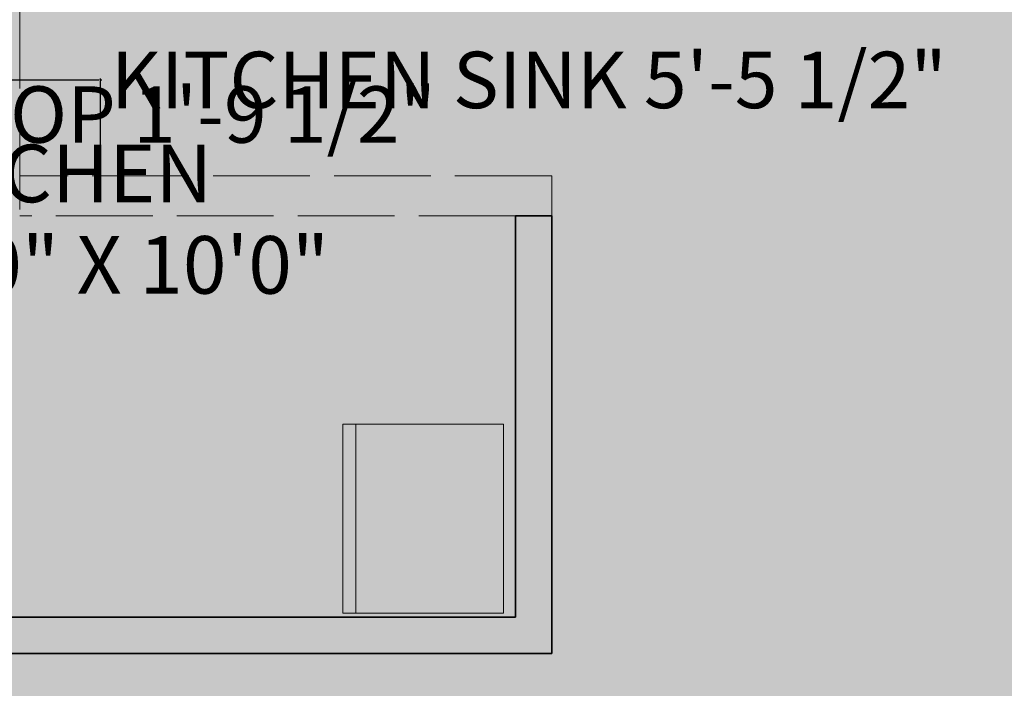
# Model space of a CAD drawing. Units: inches. Extents: x 1316 to 1777, y 813 to 1650.
# Tile 7 of 22: x 1445 to 1567, y 1237 to 1319. Entities that reach past the tile are written whole.
import ezdxf

# ---------------------------------------------------------------- set-up
doc = ezdxf.new("R2010")
doc.units = ezdxf.units.IN
doc.header["$MEASUREMENT"] = 0
doc.linetypes.add('ACAD_ISO02W100', pattern=[15, 12, -3])
for name, color, linetype, lineweight in [('A-ANNO-DIMS', 2, 'Continuous', 18), ('A-AREA-IDEN', 7, 'Continuous', 18), ('A-EQPM', 8, 'Continuous', 18), ('A-EQPM-PATT', 252, 'Continuous', 13), ('A-WALL-OVHD', 250, 'ACAD_ISO02W100', 18), ('A-WALL-PATT', 250, 'Continuous', 13), ('walls', 250, 'Continuous', 35)]:
    doc.layers.add(name, color=color, linetype=linetype, lineweight=lineweight)
doc.layers.add('A-FLOR-PATT', color=254, linetype='Continuous', lineweight=13, true_color=0xfeeab9)
doc.styles.get("Standard").update_dxf_attribs({"font": 'arial.ttf'})
doc.dimstyles.get("Standard").update_dxf_attribs({"dimtxt": 7, "dimasz": 0.18, "dimexe": 0.18, "dimexo": 0.0625, "dimgap": 0.09, "dimtad": 0, "dimtih": 1, "dimtoh": 1, "dimzin": 0, "dimdsep": 46, "dimlunit": 3, "dimtxsty": 'Standard', "dimcen": 0.09, "dimadec": 0, "dimazin": 0, "dimtfac": 1, "dimtofl": 0, "dimtmove": 0, "dimatfit": 3, "dimfxl": 1, "dimtolj": 1, "dimtzin": 0, "dimarcsym": 0})

# ---------------------------------------------------------------- blocks, each defined once
blk = doc.blocks.new('*D40')
at = {"layer": 'A-ANNO-DIMS', "color": 0, "lineweight": -2, "transparency": 16777216}
for p, q in [((1388.84, 1302.16), (1388.84, 1312.14)), ((1389.02, 1311.96), (1454.4, 1311.96)), ((1454.58, 1302.16), (1454.58, 1312.14)), ((1454.58, 1311.96), (1454.76, 1311.96))]:
    blk.add_line(p, q, dxfattribs=at)
at = {"layer": 'A-ANNO-DIMS', "color": 0, "transparency": 16777216}
for points in [[(1389.02, 1311.99), (1389.02, 1311.93), (1388.84, 1311.96)], [(1454.4, 1311.99), (1454.4, 1311.93), (1454.58, 1311.96)]]:
    blk.add_solid(points, dxfattribs=at)
at = {"layer": 'Defpoints', "color": 0, "transparency": 16777216}
for p in [(1454.58, 1311.96), (1388.84, 1302.1), (1454.58, 1302.1)]:
    blk.add_point(p, dxfattribs=at)
at = {"layer": 'A-ANNO-DIMS', "color": 0, "transparency": 16777216, "insert": (1507.74, 1311.96), "char_height": 7, "attachment_point": 5}
blk.add_mtext('\\A1;KITCHEN SINK 5\'-5 1/2"', dxfattribs=at)
blk = doc.blocks.new('*D42')
at = {"layer": 'A-ANNO-DIMS', "color": 0, "lineweight": -2, "transparency": 16777216}
for p, q in [((1388.61, 1310.85), (1388.61, 1307.49)), ((1410.21, 1310.85), (1410.21, 1307.49)), ((1388.79, 1307.67), (1410.03, 1307.67)), ((1410.21, 1307.67), (1410.39, 1307.67))]:
    blk.add_line(p, q, dxfattribs=at)
at = {"layer": 'A-ANNO-DIMS', "color": 0, "transparency": 16777216}
for points in [[(1388.79, 1307.7), (1388.79, 1307.64), (1388.61, 1307.67)], [(1410.03, 1307.7), (1410.03, 1307.64), (1410.21, 1307.67)]]:
    blk.add_solid(points, dxfattribs=at)
at = {"layer": 'Defpoints', "color": 0, "transparency": 16777216}
for p in [(1388.61, 1310.91), (1410.21, 1310.91), (1410.21, 1307.67)]:
    blk.add_point(p, dxfattribs=at)
at = {"layer": 'A-ANNO-DIMS', "color": 0, "transparency": 16777216, "insert": (1453.71, 1307.67), "char_height": 7, "attachment_point": 5}
blk.add_mtext('\\A1;COOKTOP 1\'-9 1/2"', dxfattribs=at)

msp = doc.modelspace()

# ---------------------------------------------------------------- hatches: boundary and pattern name
at = {"layer": 'A-EQPM-PATT'}
h = msp.add_hatch(color=256, dxfattribs=at)
h.dxf.hatch_style = 1
h.paths.add_polyline_path([(1504.59, 1269.305), (1486.26, 1269.305), (1486.26, 1245.841), (1504.59, 1245.841)])
h.paths.add_polyline_path([(1486.26, 1269.305), (1484.665, 1269.305), (1484.665, 1245.841), (1486.26, 1245.841)])
h = msp.add_hatch(color=256, dxfattribs=at)
h.dxf.hatch_style = 1
h.paths.add_polyline_path([(1506.155, 1265.562), (1504.59, 1265.562), (1504.59, 1250.33), (1506.155, 1250.33)])
at = {"layer": 'A-FLOR-PATT'}
h = msp.add_hatch(color=256, dxfattribs=at)
h.dxf.hatch_style = 1
h.paths.add_polyline_path([(1567.673, 1281.369), (1651.673, 1281.369), (1651.673, 1365.369), (1597.673, 1365.369), (1597.673, 1429.869), (1570.345, 1429.869), (1570.345, 1471.869), (1510.345, 1471.869), (1510.345, 1429.869), (1444.564, 1429.869), (1444.564, 1322.882), (1444.564, 1300.088), (1510.564, 1300.088), (1510.564, 1295.094), (1510.564, 1240.869), (1386.064, 1240.869), (1386.064, 1171.185), (1400.961, 1171.185), (1400.961, 1106.742), (1386.064, 1106.742), (1386.064, 1072.869), (1510.564, 1072.869), (1510.564, 1040.173), (1541.068, 1040.173, -0.367085), (1572.764, 1069.547), (1572.764, 1069.579), (1574.225, 1069.579), (1574.225, 1040.173), (1616.037, 1040.173), (1616.037, 1086.627), (1616.037, 1103.705), (1613.066, 1105.235), (1616.037, 1106.686), (1616.037, 1123.869), (1567.673, 1123.869)])
h.paths.add_polyline_path([(1508.987, 1198.018), (1511.117, 1198.018), (1511.117, 1200.148), (1532.595, 1200.148), (1532.595, 1198.018), (1534.725, 1198.018), (1534.725, 1176.008), (1530.465, 1176.008), (1530.465, 1176.718), (1513.247, 1176.718), (1513.247, 1176.008), (1508.987, 1176.008)], flags=16)
h.paths.add_polyline_path([(1505.979, 1151.315), (1521.504, 1151.315), (1521.504, 1123.623), (1505.979, 1123.623)], flags=16)
h.paths.add_polyline_path([(1507.734, 1150.101, -1), (1506.932, 1150.101, -1)], flags=0)
h.paths.add_polyline_path([(1512.288, 1138.353), (1512.28, 1138.392), (1512.219, 1138.376)], flags=0)
h.paths.add_polyline_path([(1511.539, 1138.926), (1511.802, 1138.967), (1511.817, 1139.27), (1511.607, 1139.246)], flags=0)
h.paths.add_polyline_path([(1513.745, 1140.234), (1513.68, 1139.885), (1514.014, 1140.045), (1513.855, 1140.308)], flags=0)
h.paths.add_polyline_path([(1513.759, 1139.089), (1514.005, 1139.255), (1513.807, 1139.483), (1513.564, 1139.327)], flags=0)
h.paths.add_polyline_path([(1514.219, 1138.385), (1514.336, 1138.33), (1514.544, 1138.32), (1514.802, 1138.874), (1514.451, 1138.716)], flags=0)
h.paths.add_polyline_path([(1514.577, 1137.439), (1514.573, 1137.4), (1514.699, 1137.4), (1514.696, 1137.402)], flags=0)
h.paths.add_polyline_path([(1512.26, 1136.199), (1512.199, 1136.399), (1512.032, 1136.325), (1512.095, 1136.101), (1512.257, 1136.192)], flags=0)
h.paths.add_polyline_path([(1512.644, 1137.274), (1512.356, 1137.23), (1512.432, 1137.049), (1512.703, 1137.093)], flags=0)
h.paths.add_polyline_path([(1513.049, 1137.593), (1512.979, 1137.8), (1512.843, 1137.757), (1512.887, 1137.556)], flags=0)
h.paths.add_polyline_path([(1513.269, 1138.556), (1513.571, 1137.962), (1513.459, 1136.814), (1513.212, 1137.878), (1513.032, 1138.443)], flags=0)
h.paths.add_polyline_path([(1514.891, 1136.377), (1514.696, 1136.401), (1514.683, 1136.246), (1514.87, 1136.165)], flags=0)
h.paths.add_polyline_path([(1514.142, 1137.293), (1514.047, 1136.743), (1514.27, 1136.751), (1514.328, 1137.265)], flags=0)
h.paths.add_polyline_path([(1515.362, 1138.976), (1515.334, 1138.638), (1515.596, 1138.588), (1515.627, 1138.932)], flags=0)
h.paths.add_polyline_path([(1537.285, 1177.912), (1537.995, 1177.912), (1537.995, 1195.13), (1537.285, 1195.13), (1537.285, 1199.39), (1559.295, 1199.39), (1559.295, 1197.26), (1561.425, 1197.26), (1561.425, 1175.782), (1559.295, 1175.782), (1559.295, 1173.652), (1559.379, 1173.652), (1559.379, 1171.514), (1561.517, 1171.514), (1561.517, 1098.819), (1559.379, 1098.819), (1559.379, 1096.68), (1537.285, 1096.68), (1537.285, 1100.957), (1537.997, 1100.957), (1537.997, 1169.376), (1537.285, 1169.376), (1537.285, 1173.652)], flags=16)
h.paths.add_polyline_path([(1518.623, 1345.565), (1519.133, 1345.48), (1519.133, 1345.485), (1518.623, 1345.567)], flags=16)
h.paths.add_polyline_path([(1518.798, 1374.15), (1519.308, 1374.064), (1519.308, 1374.069), (1518.798, 1374.152)], flags=16)
h.paths.add_polyline_path([(1537.764, 1413.501), (1537.678, 1412.991), (1537.683, 1412.991), (1537.766, 1413.501)], flags=16)
h.paths.add_polyline_path([(1572.905, 1373.821), (1573.927, 1373.975), (1574.027, 1390.309), (1573.007, 1390.475), (1573.007, 1390.475)], flags=16)
h.paths.add_polyline_path([(1572.73, 1345.237), (1573.752, 1345.39), (1573.852, 1361.724), (1572.832, 1361.89), (1572.832, 1361.89)], flags=16)
h.paths.add_polyline_path([(1537.211, 1322.643), (1537.364, 1321.621), (1553.698, 1321.521), (1553.864, 1322.541)], flags=16)
h.paths.add_polyline_path([(1535.908, 1331.328), (1527.214, 1331.382), (1527.664, 1404.885), (1564.416, 1404.66), (1563.966, 1331.157), (1555.273, 1331.21), (1553.947, 1323.051), (1537.134, 1323.154)], flags=16)
h.paths.add_polyline_path([(1536.15, 1336.503), (1536.235, 1337.572), (1536.323, 1338.628), (1536.411, 1339.663), (1536.495, 1340.67), (1536.574, 1341.66), (1536.648, 1342.648), (1536.717, 1343.649), (1536.78, 1344.678), (1536.837, 1345.75), (1536.913, 1347.475), (1536.93, 1348.082), (1536.867, 1346.314), (1536.754, 1344.188), (1536.619, 1342.219), (1536.495, 1340.67), (1536.411, 1339.663), (1536.323, 1338.628), (1536.235, 1337.572), (1536.15, 1336.503), (1536.071, 1335.432), (1536.002, 1334.37), (1535.917, 1332.754), (1535.909, 1332.308), (1535.964, 1333.78), (1536.071, 1335.432)], flags=0)
h.paths.add_polyline_path([(1540.412, 1338.345), (1540.539, 1339.037), (1540.667, 1339.758), (1540.798, 1340.518), (1540.93, 1341.325), (1541.063, 1342.187), (1541.196, 1343.109), (1541.326, 1344.085), (1541.45, 1345.102), (1541.566, 1346.15), (1541.669, 1347.219), (1541.758, 1348.296), (1541.829, 1349.371), (1541.879, 1350.434), (1541.906, 1351.476), (1541.91, 1352.5), (1541.895, 1353.512), (1541.861, 1354.518), (1541.812, 1355.524), (1541.749, 1356.537), (1541.674, 1357.561), (1541.551, 1359.062), (1541.495, 1359.67), (1541.589, 1358.603), (1541.721, 1356.977), (1541.846, 1354.98), (1541.912, 1352.982), (1541.903, 1350.951), (1541.806, 1348.87), (1541.628, 1346.713), (1541.396, 1344.612), (1541.135, 1342.656), (1540.872, 1340.947), (1540.617, 1339.466), (1540.412, 1338.345), (1540.288, 1337.675), (1540.166, 1337.018), (1540.049, 1336.365), (1539.937, 1335.71), (1539.837, 1335.055), (1539.758, 1334.403), (1539.709, 1333.756), (1539.697, 1333.12), (1539.751, 1332.162), (1539.822, 1331.89), (1539.691, 1332.775), (1539.714, 1334.035), (1539.867, 1335.303), (1540.085, 1336.577), (1540.288, 1337.675)], flags=0)
h.paths.add_polyline_path([(1545.599, 1331.584), (1545.601, 1331.617), (1545.614, 1331.689), (1545.737, 1332.197), (1545.767, 1332.332), (1545.84, 1332.681), (1545.925, 1333.114), (1546.016, 1333.614), (1546.108, 1334.164), (1546.196, 1334.748), (1546.276, 1335.349), (1546.342, 1335.952), (1546.388, 1336.539), (1546.412, 1337.098), (1546.414, 1337.632), (1546.395, 1338.145), (1546.359, 1338.645), (1546.306, 1339.137), (1546.24, 1339.627), (1546.161, 1340.121), (1546.073, 1340.625), (1545.888, 1341.63), (1545.718, 1342.621), (1545.547, 1343.945), (1545.432, 1345.534), (1545.404, 1347.402), (1545.418, 1348.013), (1545.411, 1346.957), (1545.425, 1345.988), (1545.463, 1345.105), (1545.521, 1344.301), (1545.596, 1343.566), (1545.683, 1342.892), (1545.778, 1342.27), (1545.877, 1341.691), (1545.977, 1341.145), (1546.133, 1340.297), (1546.327, 1339.075), (1546.434, 1337.615), (1546.377, 1336.279), (1546.246, 1335.079), (1546.032, 1333.665), (1545.84, 1332.681), (1545.767, 1332.332)], flags=0)
h.paths.add_polyline_path([(1551.803, 1337.656), (1551.963, 1338.25), (1552.102, 1338.801), (1552.225, 1339.338), (1552.331, 1339.865), (1552.418, 1340.377), (1552.487, 1340.873), (1552.536, 1341.348), (1552.563, 1341.801), (1552.569, 1342.228), (1552.551, 1342.627), (1552.51, 1342.995), (1552.446, 1343.333), (1552.363, 1343.646), (1552.261, 1343.937), (1552.144, 1344.207), (1552.012, 1344.461), (1551.868, 1344.7), (1551.746, 1344.882), (1550.887, 1346.052), (1550.428, 1347.126), (1550.183, 1348.353), (1550.048, 1349.632), (1549.978, 1351.224), (1549.974, 1353.141), (1549.989, 1353.748), (1549.975, 1352.682), (1549.977, 1351.708), (1549.996, 1350.825), (1550.031, 1350.027), (1550.082, 1349.31), (1550.15, 1348.669), (1550.234, 1348.098), (1550.335, 1347.593), (1550.452, 1347.149), (1550.584, 1346.76), (1550.73, 1346.419), (1550.887, 1346.117), (1551.05, 1345.848), (1551.217, 1345.602), (1551.386, 1345.372), (1551.553, 1345.151), (1552, 1344.537), (1552.454, 1343.495), (1552.591, 1342.266), (1552.509, 1340.905), (1552.246, 1339.367), (1551.925, 1338.101), (1551.619, 1336.984), (1551.406, 1336.2), (1551.01, 1334.699), (1550.877, 1334.155), (1551.264, 1335.677), (1551.619, 1336.984)], flags=0)
h.paths.add_polyline_path([(1558.642, 1348.348), (1558.795, 1348.811), (1558.918, 1349.215), (1559.008, 1349.575), (1559.061, 1349.904), (1559.076, 1350.214), (1559.054, 1350.506), (1559.001, 1350.776), (1558.919, 1351.021), (1558.814, 1351.239), (1558.688, 1351.425), (1558.546, 1351.578), (1558.392, 1351.694), (1558.229, 1351.772), (1558.059, 1351.812), (1557.882, 1351.819), (1557.701, 1351.794), (1557.515, 1351.742), (1557.327, 1351.665), (1557.136, 1351.566), (1556.944, 1351.448), (1556.752, 1351.315), (1556.742, 1351.307), (1556.175, 1350.878), (1555.982, 1350.741), (1555.79, 1350.618), (1555.103, 1350.248), (1554.019, 1350.696), (1553.658, 1351.734), (1553.592, 1352.861), (1553.705, 1354.248), (1553.753, 1354.657), (1553.685, 1354.004), (1553.638, 1353.425), (1553.615, 1352.918), (1553.615, 1352.476), (1553.637, 1352.094), (1553.681, 1351.766), (1553.745, 1351.485), (1553.828, 1351.246), (1553.929, 1351.043), (1554.048, 1350.87), (1554.182, 1350.722), (1554.33, 1350.599), (1554.491, 1350.501), (1554.662, 1350.43), (1554.841, 1350.388), (1555.026, 1350.374), (1555.215, 1350.39), (1555.406, 1350.437), (1555.598, 1350.514), (1555.79, 1350.618), (1555.982, 1350.741), (1556.175, 1350.878), (1556.367, 1351.024), (1556.559, 1351.171), (1556.752, 1351.315), (1556.944, 1351.448), (1557.136, 1351.566), (1557.327, 1351.665), (1558.043, 1351.957), (1558.894, 1351.316), (1559.137, 1350.09), (1558.886, 1349.087), (1558.642, 1348.348), (1558.463, 1347.812), (1558.261, 1347.187), (1558.039, 1346.459), (1557.677, 1345.175), (1557.549, 1344.636), (1557.909, 1346.03), (1558.329, 1347.408)], flags=0)
h.paths.add_polyline_path([(1562.145, 1353.919), (1562.25, 1354.68), (1562.341, 1355.344), (1562.416, 1355.924), (1562.475, 1356.431), (1562.518, 1356.872), (1562.544, 1357.254), (1562.554, 1357.582), (1562.548, 1357.862), (1562.525, 1358.1), (1562.486, 1358.303), (1562.432, 1358.476), (1562.361, 1358.624), (1562.277, 1358.748), (1562.18, 1358.848), (1562.073, 1358.925), (1561.958, 1358.977), (1561.837, 1359.006), (1561.711, 1359.011), (1561.584, 1358.992), (1561.456, 1358.949), (1561.342, 1358.895), (1560.78, 1358.554), (1560.631, 1358.473), (1560.474, 1358.403), (1560.311, 1358.348), (1559.637, 1358.207), (1558.973, 1358.904), (1558.816, 1360.002), (1558.804, 1361.236), (1558.83, 1361.674), (1558.807, 1360.917), (1558.813, 1360.297), (1558.845, 1359.795), (1558.902, 1359.397), (1558.982, 1359.087), (1559.082, 1358.849), (1559.2, 1358.666), (1559.334, 1358.525), (1559.482, 1358.421), (1559.639, 1358.351), (1559.804, 1358.311), (1559.973, 1358.3), (1560.143, 1358.313), (1560.311, 1358.348), (1560.474, 1358.403), (1560.631, 1358.473), (1560.78, 1358.554), (1560.923, 1358.641), (1561.061, 1358.729), (1561.196, 1358.813), (1561.382, 1358.92), (1561.342, 1358.895), (1561.972, 1359.194), (1562.536, 1358.367), (1562.56, 1357.311), (1562.455, 1356.226), (1562.323, 1355.206), (1562.145, 1353.919), (1562.026, 1353.049), (1561.815, 1351.457), (1561.752, 1350.933), (1561.948, 1352.479)], flags=0)
h.paths.add_polyline_path([(1572.764, 1069.547, 0.367085), (1541.068, 1040.173), (1572.764, 1040.173)], flags=17)
h.paths.add_polyline_path([(1572.764, 1040.173), (1541.068, 1040.173, 0.0299535), (1540.829, 1036.182), (1540.829, 1031.173), (1574.225, 1031.173), (1574.225, 1036.182), (1572.764, 1036.182)])
h = msp.add_hatch(color=256, dxfattribs=at)
h.dxf.hatch_style = 1
h.paths.add_polyline_path([(1506.064, 1295.094), (1444.564, 1295.094), (1444.564, 1322.882), (1440.064, 1322.882), (1440.064, 1346.929), (1412.858, 1346.929), (1412.858, 1245.369), (1506.064, 1245.369)])
h.paths.add_polyline_path([(1484.665, 1269.305), (1504.59, 1269.305), (1504.59, 1245.841), (1484.665, 1245.841)], flags=16)
h.paths.add_polyline_path([(1510.564, 1300.088), (1444.564, 1300.088), (1444.564, 1295.094), (1506.064, 1295.094), (1510.564, 1295.094)])
at = {"layer": 'A-WALL-PATT'}
h = msp.add_hatch(color=256, dxfattribs=at)
h.dxf.hatch_style = 1
h.paths.add_polyline_path([(1713.173, 1281.369), (1656.173, 1281.369), (1656.173, 1298.258), (1651.673, 1298.258), (1651.673, 1281.369), (1567.673, 1281.369), (1567.673, 1266.995), (1572.173, 1266.995), (1572.173, 1276.869), (1704.173, 1276.869), (1704.173, 1132.869), (1608.64, 1132.869), (1608.64, 1123.869), (1704.173, 1123.869), (1704.173, 1040.173), (1652.869, 1040.173), (1652.869, 1031.173), (1713.173, 1031.173), (1713.173, 1040.173)])
h.paths.add_polyline_path([(1572.173, 1237.955), (1567.673, 1237.955), (1567.673, 1123.869), (1583.146, 1123.869), (1583.146, 1132.869), (1572.173, 1132.869)], flags=17)
h.paths.add_polyline_path([(1510.345, 1566.369), (1524.171, 1566.369), (1524.171, 1571.985), (1524.171, 1575.369), (1445.955, 1575.369), (1445.955, 1566.369), (1505.845, 1566.369), (1505.845, 1469.591), (1510.345, 1469.591), (1510.345, 1471.869), (1529.081, 1471.869), (1529.081, 1476.369), (1510.345, 1476.369)])
h.paths.add_polyline_path([(1609.722, 1575.369), (1545.119, 1575.369), (1545.119, 1566.369), (1570.345, 1566.369), (1570.345, 1476.369), (1562.477, 1476.369), (1562.477, 1471.869), (1570.345, 1471.869), (1570.345, 1469.591), (1574.845, 1469.591), (1574.845, 1566.369), (1609.722, 1566.369)])
h.paths.add_polyline_path([(1713.173, 1575.369), (1655.233, 1575.369), (1655.233, 1566.369), (1704.173, 1566.369), (1704.173, 1434.369), (1574.845, 1434.369), (1574.845, 1440.551), (1574.701, 1440.551), (1570.345, 1440.551), (1570.345, 1429.869), (1597.673, 1429.869), (1597.673, 1408.281), (1602.173, 1408.281), (1602.173, 1429.869), (1704.173, 1429.869), (1704.173, 1410.704), (1707.375, 1410.704), (1713.173, 1410.704)])
h.paths.add_polyline_path([(1713.173, 1383.676), (1704.173, 1383.676), (1704.173, 1369.869), (1602.173, 1369.869), (1602.173, 1379.241), (1597.673, 1379.241), (1597.673, 1365.369), (1713.173, 1365.369)])
h.paths.add_polyline_path([(1444.564, 1429.869), (1510.345, 1429.869), (1510.345, 1440.551), (1505.845, 1440.551), (1505.845, 1434.369), (1386.064, 1434.369), (1386.064, 1566.369), (1400.445, 1566.369), (1400.445, 1575.369), (1377.064, 1575.369), (1377.064, 1412.813), (1380.509, 1412.813), (1386.064, 1412.813), (1386.064, 1429.869), (1440.064, 1429.869), (1440.064, 1401.229), (1444.564, 1401.229)])
h.paths.add_polyline_path([(1444.564, 1372.189), (1440.064, 1372.189), (1440.064, 1369.869), (1386.064, 1369.869), (1386.064, 1378.758), (1377.064, 1378.758), (1377.064, 1349.201), (1381.118, 1349.201), (1386.064, 1349.201), (1386.064, 1365.369), (1440.064, 1365.369), (1440.064, 1322.882), (1444.564, 1322.882)])
h.paths.add_polyline_path([(1510.564, 1295.094), (1506.064, 1295.094), (1506.064, 1245.369), (1386.064, 1245.369), (1386.064, 1272.582), (1377.064, 1272.582), (1377.064, 1212.905), (1380.1, 1212.905), (1386.064, 1212.905), (1386.064, 1240.869), (1510.564, 1240.869)])
h.paths.add_polyline_path([(1386.064, 1163.761), (1377.064, 1163.761), (1377.064, 1063.869), (1419.363, 1063.869), (1419.363, 1072.869), (1386.064, 1072.869)])
h.paths.add_polyline_path([(1510.564, 1072.869), (1469.381, 1072.869), (1469.381, 1063.869), (1501.564, 1063.869), (1501.564, 1033.023), (1501.564, 1031.173), (1540.829, 1031.173), (1540.829, 1036.182, -0.0299535), (1541.068, 1040.173), (1510.564, 1040.173)])
h.paths.add_polyline_path([(1607.369, 1040.173), (1574.225, 1040.173), (1574.225, 1036.182), (1574.225, 1031.173), (1607.369, 1031.173)], flags=17)
h.paths.add_polyline_path([(1637.054, 1040.173), (1624.706, 1040.173), (1624.706, 1031.173), (1637.054, 1031.173)], flags=17)

# ---------------------------------------------------------------- linework, layer by layer
at = {"layer": 'A-EQPM'}
for p, q in [((1484.665, 1245.841), (1484.665, 1269.305)), ((1484.665, 1269.305), (1504.59, 1269.305)), ((1486.26, 1245.841), (1486.26, 1269.305)), ((1504.59, 1269.305), (1504.59, 1245.841)), ((1504.59, 1245.841), (1484.665, 1245.841))]:
    msp.add_line(p, q, dxfattribs=at)
at = {"layer": 'A-WALL-OVHD'}
for p, q in [((1444.564, 1322.882), (1444.564, 1295.189)), ((1510.564, 1300.088), (1444.564, 1300.088)), ((1510.564, 1295.094), (1510.564, 1300.088)), ((1506.064, 1295.094), (1444.564, 1295.094))]:
    msp.add_line(p, q, dxfattribs=at)
at = {"layer": 'walls'}
for p, q in [((1506.064, 1295.094), (1506.064, 1245.369)), ((1506.064, 1295.094), (1510.564, 1295.094)), ((1510.564, 1295.094), (1510.564, 1240.869)), ((1386.064, 1245.369), (1506.064, 1245.369)), ((1386.064, 1240.869), (1510.564, 1240.869))]:
    msp.add_line(p, q, dxfattribs=at)

# ---------------------------------------------------------------- texts
at = {"layer": 'A-AREA-IDEN'}
for s, height, p in [('KITCHEN', 7.1416, (1427.365, 1296.796)), ('10\'0" X 10\'0"', 7.14165, (1425.905, 1285.462))]:
    msp.add_text(s, height=height, dxfattribs=at).set_placement(p)

# ---------------------------------------------------------------- dimensions: what is measured, and where the dimension line sits
at = {"layer": 'A-ANNO-DIMS'}
for base, p1, p2, text, picture, middle in [((1454.577, 1311.961), (1388.838, 1302.1), (1454.577, 1302.1), 'KITCHEN SINK <>', '*D40', (1507.741, 1311.961)), ((1410.21, 1307.675), (1388.61, 1310.915), (1410.21, 1310.915), 'COOKTOP <>', '*D42', (1453.708, 1307.675))]:
    dim = msp.add_linear_dim(base=base, p1=p1, p2=p2, text=text, dimstyle='Standard', override={"dimdec": 1, "dimlfac": 1, "dimrnd": 0, "dimzin": 1, "dimdsep": 46, "dimlunit": 4, "dimfrac": 2}, dxfattribs=at)
    dim.commit()
    dim.dimension.update_dxf_attribs({"geometry": picture, "text_midpoint": middle})

doc.saveas('drawing.dxf')
